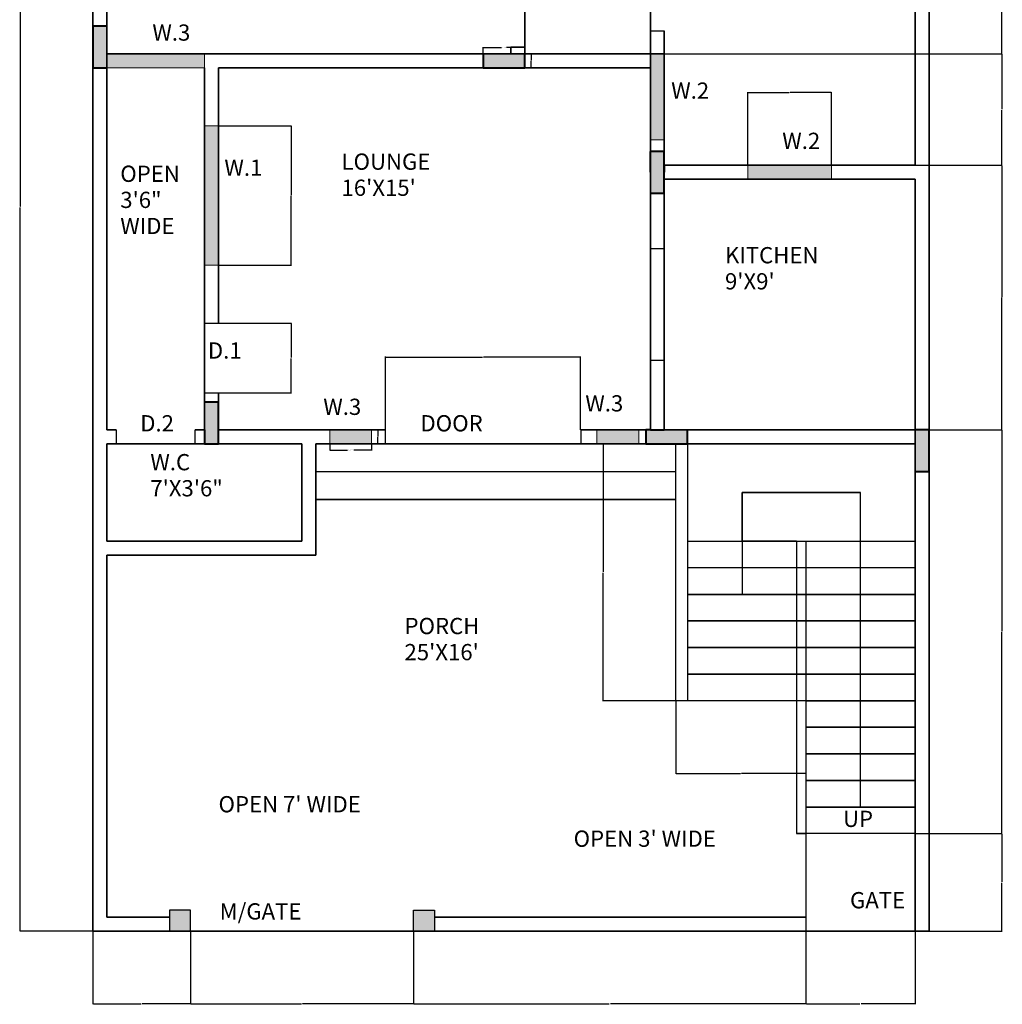
# Model space of a CAD drawing. Units: inches. Extents: x 2156 to 3149, y 1513 to 2286.
# Tile 1 of 5: x 2156 to 2579, y 1513 to 1937. Entities that reach past the tile are written whole.
import ezdxf

# ---------------------------------------------------------------- set-up
doc = ezdxf.new("R2010")
doc.units = ezdxf.units.IN
for name, color, linetype, lineweight in [('A-ANNO-DIMS', 2, 'Continuous', 18), ('A-ANNO-TEXT', 7, 'Continuous', 18), ('A-AREA-IDEN', 7, 'Continuous', 18), ('A-COLS', 7, 'Continuous', 40), ('A-COLS-PATT', 18, 'Continuous', 13), ('A-CONS', 8, 'Continuous', 9), ('A-DOOR', 3, 'Continuous', 25), ('A-FLOR-STRS', 7, 'Continuous', 25), ('A-GLAZ', 4, 'Continuous', 18), ('A-GLAZ-PATT', 252, 'Continuous', 13), ('A-SITE-GATE', 3, 'Continuous', 25), ('A-SITE-WALL', 7, 'Continuous', 35), ('A-WALL', 7, 'Continuous', 35)]:
    doc.layers.add(name, color=color, linetype=linetype, lineweight=lineweight)
doc.styles.get("Standard").update_dxf_attribs({"font": 'arial.ttf'})
doc.dimstyles.get("Standard").update_dxf_attribs({"dimtxt": 0.18, "dimasz": 0.18, "dimexe": 0.18, "dimexo": 0.0625, "dimgap": 0.09, "dimtad": 0, "dimtih": 1, "dimtoh": 1, "dimdec": 4, "dimzin": 0, "dimdsep": 46, "dimtxsty": 'Standard', "dimcen": 0.09, "dimadec": 0, "dimazin": 0, "dimtfac": 1, "dimtdec": 4, "dimtofl": 0, "dimtmove": 0, "dimatfit": 3, "dimfxl": 1, "dimtolj": 1, "dimtzin": 0, "dimarcsym": 0})

# ---------------------------------------------------------------- blocks, each defined once
blk = doc.blocks.new('COL-6X18-PLAN')
for p, q in [((6, 18), (0, 18)), ((0, 18), (0, 0)), ((0, 0), (6, 0))]:
    blk.add_line(p, q)
blk = doc.blocks.new('WIN-W3-18-PLAN')
for p, q in [((18, 6), (0, 6)), ((0, 6), (0, 0)), ((18, 0), (18, 6))]:
    blk.add_line(p, q)
blk = doc.blocks.new('*D7')
at = {"layer": 'A-ANNO-DIMS', "color": 0, "lineweight": -2, "transparency": 16777216}
for p, q in [((2355.92, 1922.6), (2355.92, 1925.42)), ((2356.1, 1925.24), (2363.81, 1925.24)), ((2373.74, 1925.24), (2366.03, 1925.24)), ((2373.92, 1922.6), (2373.92, 1925.42))]:
    blk.add_line(p, q, dxfattribs=at)
at = {"layer": 'A-ANNO-DIMS', "color": 0, "transparency": 16777216}
for points in [[(2356.1, 1925.27), (2356.1, 1925.21), (2355.92, 1925.24)], [(2373.74, 1925.27), (2373.74, 1925.21), (2373.92, 1925.24)]]:
    blk.add_solid(points, dxfattribs=at)
at = {"layer": 'Defpoints', "color": 0, "transparency": 16777216}
for p in [(2355.92, 1925.24), (2355.92, 1922.54), (2373.92, 1922.54)]:
    blk.add_point(p, dxfattribs=at)
at = {"layer": 'A-ANNO-DIMS', "color": 0, "transparency": 16777216, "insert": (2364.92, 1925.24), "char_height": 0.18, "attachment_point": 5}
blk.add_mtext('\\A1;COLUMN 18 TYP.', dxfattribs=at)
blk = doc.blocks.new('*D8')
at = {"layer": 'A-ANNO-DIMS', "color": 0, "lineweight": -2, "transparency": 16777216}
for p, q in [((2373.98, 1922.54), (2376.8, 1922.54)), ((2376.62, 1922.36), (2376.62, 1919.72)), ((2376.62, 1916.72), (2376.62, 1919.35)), ((2373.98, 1916.54), (2376.8, 1916.54))]:
    blk.add_line(p, q, dxfattribs=at)
at = {"layer": 'A-ANNO-DIMS', "color": 0, "transparency": 16777216}
for points in [[(2376.59, 1922.36), (2376.65, 1922.36), (2376.62, 1922.54)], [(2376.59, 1916.72), (2376.65, 1916.72), (2376.62, 1916.54)]]:
    blk.add_solid(points, dxfattribs=at)
at = {"layer": 'Defpoints', "color": 0, "transparency": 16777216}
for p in [(2373.92, 1922.54), (2376.62, 1922.54), (2373.92, 1916.54)]:
    blk.add_point(p, dxfattribs=at)
at = {"layer": 'A-ANNO-DIMS', "color": 0, "transparency": 16777216, "insert": (2376.62, 1919.54), "char_height": 0.18, "attachment_point": 5}
blk.add_mtext('\\A1;6 TYP.', dxfattribs=at)
blk = doc.blocks.new('*D11')
at = {"layer": 'A-ANNO-DIMS', "color": 0, "lineweight": -2, "transparency": 16777216}
for p, q in [((2289.92, 1754.47), (2289.92, 1751.66)), ((2307.92, 1754.47), (2307.92, 1751.66)), ((2290.1, 1751.84), (2297.58, 1751.84)), ((2307.74, 1751.84), (2300.26, 1751.84))]:
    blk.add_line(p, q, dxfattribs=at)
at = {"layer": 'A-ANNO-DIMS', "color": 0, "transparency": 16777216}
for points in [[(2290.1, 1751.87), (2290.1, 1751.81), (2289.92, 1751.84)], [(2307.74, 1751.87), (2307.74, 1751.81), (2307.92, 1751.84)]]:
    blk.add_solid(points, dxfattribs=at)
at = {"layer": 'Defpoints', "color": 0, "transparency": 16777216}
for p in [(2289.92, 1754.54), (2307.92, 1754.54), (2307.92, 1751.84)]:
    blk.add_point(p, dxfattribs=at)
at = {"layer": 'A-ANNO-DIMS', "color": 0, "transparency": 16777216, "insert": (2298.92, 1751.84), "char_height": 0.18, "attachment_point": 5}
blk.add_mtext('\\A1;W3 WINDOW 18 TYP.', dxfattribs=at)
blk = doc.blocks.new('*D12')
at = {"layer": 'A-ANNO-DIMS', "color": 0, "lineweight": -2, "transparency": 16777216}
for p, q in [((2307.98, 1760.54), (2310.8, 1760.54)), ((2310.62, 1760.36), (2310.62, 1757.72)), ((2310.62, 1754.72), (2310.62, 1757.35)), ((2307.98, 1754.54), (2310.8, 1754.54))]:
    blk.add_line(p, q, dxfattribs=at)
at = {"layer": 'A-ANNO-DIMS', "color": 0, "transparency": 16777216}
for points in [[(2310.59, 1760.36), (2310.65, 1760.36), (2310.62, 1760.54)], [(2310.59, 1754.72), (2310.65, 1754.72), (2310.62, 1754.54)]]:
    blk.add_solid(points, dxfattribs=at)
at = {"layer": 'Defpoints', "color": 0, "transparency": 16777216}
for p in [(2307.92, 1760.54), (2310.62, 1760.54), (2307.92, 1754.54)]:
    blk.add_point(p, dxfattribs=at)
at = {"layer": 'A-ANNO-DIMS', "color": 0, "transparency": 16777216, "insert": (2310.62, 1757.54), "char_height": 0.18, "attachment_point": 5}
blk.add_mtext('\\A1;6 TYP.', dxfattribs=at)
blk = doc.blocks.new('*D20')
at = {"layer": 'A-ANNO-DIMS', "color": 0, "lineweight": -2, "transparency": 16777216}
for p, q in [((2187.92, 1544.47), (2187.92, 1513.01)), ((2229.92, 1544.47), (2229.92, 1513.01)), ((2188.1, 1513.19), (2208.7, 1513.19)), ((2229.74, 1513.19), (2209.14, 1513.19))]:
    blk.add_line(p, q, dxfattribs=at)
at = {"layer": 'A-ANNO-DIMS', "color": 0, "transparency": 16777216}
for points in [[(2188.1, 1513.22), (2188.1, 1513.16), (2187.92, 1513.19)], [(2229.74, 1513.22), (2229.74, 1513.16), (2229.92, 1513.19)]]:
    blk.add_solid(points, dxfattribs=at)
at = {"layer": 'Defpoints', "color": 0, "transparency": 16777216}
for p in [(2187.92, 1544.54), (2229.92, 1544.54), (2229.92, 1513.19)]:
    blk.add_point(p, dxfattribs=at)
at = {"layer": 'A-ANNO-DIMS', "color": 0, "transparency": 16777216, "insert": (2208.92, 1513.19), "char_height": 0.18, "attachment_point": 5}
blk.add_mtext('\\A1;42', dxfattribs=at)
blk = doc.blocks.new('*D21')
at = {"layer": 'A-ANNO-DIMS', "color": 0, "lineweight": -2, "transparency": 16777216}
for p, q in [((2229.92, 1544.47), (2229.92, 1513.01)), ((2325.92, 1544.47), (2325.92, 1513.01)), ((2230.1, 1513.19), (2277.7, 1513.19)), ((2325.74, 1513.19), (2278.14, 1513.19))]:
    blk.add_line(p, q, dxfattribs=at)
at = {"layer": 'A-ANNO-DIMS', "color": 0, "transparency": 16777216}
for points in [[(2230.1, 1513.22), (2230.1, 1513.16), (2229.92, 1513.19)], [(2325.74, 1513.22), (2325.74, 1513.16), (2325.92, 1513.19)]]:
    blk.add_solid(points, dxfattribs=at)
at = {"layer": 'Defpoints', "color": 0, "transparency": 16777216}
for p in [(2229.92, 1544.54), (2325.92, 1544.54), (2325.92, 1513.19)]:
    blk.add_point(p, dxfattribs=at)
at = {"layer": 'A-ANNO-DIMS', "color": 0, "transparency": 16777216, "insert": (2277.92, 1513.19), "char_height": 0.18, "attachment_point": 5}
blk.add_mtext('\\A1;96', dxfattribs=at)
blk = doc.blocks.new('*D22')
at = {"layer": 'A-ANNO-DIMS', "color": 0, "lineweight": -2, "transparency": 16777216}
for p, q in [((2325.92, 1544.47), (2325.92, 1513.01)), ((2494.92, 1544.47), (2494.92, 1513.01)), ((2326.1, 1513.19), (2410.14, 1513.19)), ((2494.74, 1513.19), (2410.7, 1513.19))]:
    blk.add_line(p, q, dxfattribs=at)
at = {"layer": 'A-ANNO-DIMS', "color": 0, "transparency": 16777216}
for points in [[(2326.1, 1513.22), (2326.1, 1513.16), (2325.92, 1513.19)], [(2494.74, 1513.22), (2494.74, 1513.16), (2494.92, 1513.19)]]:
    blk.add_solid(points, dxfattribs=at)
at = {"layer": 'Defpoints', "color": 0, "transparency": 16777216}
for p in [(2325.92, 1544.54), (2494.92, 1544.54), (2494.92, 1513.19)]:
    blk.add_point(p, dxfattribs=at)
at = {"layer": 'A-ANNO-DIMS', "color": 0, "transparency": 16777216, "insert": (2410.42, 1513.19), "char_height": 0.18, "attachment_point": 5}
blk.add_mtext('\\A1;169', dxfattribs=at)
blk = doc.blocks.new('*D23')
at = {"layer": 'A-ANNO-DIMS', "color": 0, "lineweight": -2, "transparency": 16777216}
for p, q in [((2494.92, 1544.47), (2494.92, 1513.01)), ((2541.92, 1544.47), (2541.92, 1513.01)), ((2495.1, 1513.19), (2518.2, 1513.19)), ((2541.74, 1513.19), (2518.64, 1513.19))]:
    blk.add_line(p, q, dxfattribs=at)
at = {"layer": 'A-ANNO-DIMS', "color": 0, "transparency": 16777216}
for points in [[(2495.1, 1513.22), (2495.1, 1513.16), (2494.92, 1513.19)], [(2541.74, 1513.22), (2541.74, 1513.16), (2541.92, 1513.19)]]:
    blk.add_solid(points, dxfattribs=at)
at = {"layer": 'Defpoints', "color": 0, "transparency": 16777216}
for p in [(2494.92, 1544.54), (2541.92, 1544.54), (2541.92, 1513.19)]:
    blk.add_point(p, dxfattribs=at)
at = {"layer": 'A-ANNO-DIMS', "color": 0, "transparency": 16777216, "insert": (2518.42, 1513.19), "char_height": 0.18, "attachment_point": 5}
blk.add_mtext('\\A1;47', dxfattribs=at)
blk = doc.blocks.new('*D24')
at = {"layer": 'A-ANNO-DIMS', "color": 0, "lineweight": -2, "transparency": 16777216}
for p, q in [((2187.86, 2168.54), (2156.39, 2168.54)), ((2156.57, 2168.36), (2156.57, 1856.72)), ((2156.57, 1544.72), (2156.57, 1856.35)), ((2187.86, 1544.54), (2156.39, 1544.54))]:
    blk.add_line(p, q, dxfattribs=at)
at = {"layer": 'A-ANNO-DIMS', "color": 0, "transparency": 16777216}
for points in [[(2156.54, 2168.36), (2156.6, 2168.36), (2156.57, 2168.54)], [(2156.54, 1544.72), (2156.6, 1544.72), (2156.57, 1544.54)]]:
    blk.add_solid(points, dxfattribs=at)
at = {"layer": 'Defpoints', "color": 0, "transparency": 16777216}
for p in [(2156.57, 2168.54), (2187.92, 2168.54), (2187.92, 1544.54)]:
    blk.add_point(p, dxfattribs=at)
at = {"layer": 'A-ANNO-DIMS', "color": 0, "transparency": 16777216, "insert": (2156.57, 1856.54), "char_height": 0.18, "attachment_point": 5}
blk.add_mtext('\\A1;624', dxfattribs=at)
blk = doc.blocks.new('*D25')
at = {"layer": 'A-ANNO-DIMS', "color": 0, "lineweight": -2, "transparency": 16777216}
for p, q in [((2541.98, 1586.54), (2579.45, 1586.54)), ((2579.27, 1586.36), (2579.27, 1565.72)), ((2579.27, 1544.72), (2579.27, 1565.36)), ((2547.98, 1544.54), (2579.45, 1544.54))]:
    blk.add_line(p, q, dxfattribs=at)
at = {"layer": 'A-ANNO-DIMS', "color": 0, "transparency": 16777216}
for points in [[(2579.24, 1586.36), (2579.3, 1586.36), (2579.27, 1586.54)], [(2579.24, 1544.72), (2579.3, 1544.72), (2579.27, 1544.54)]]:
    blk.add_solid(points, dxfattribs=at)
at = {"layer": 'Defpoints', "color": 0, "transparency": 16777216}
for p in [(2541.92, 1586.54), (2579.27, 1586.54), (2547.92, 1544.54)]:
    blk.add_point(p, dxfattribs=at)
at = {"layer": 'A-ANNO-DIMS', "color": 0, "transparency": 16777216, "insert": (2579.27, 1565.54), "char_height": 0.18, "attachment_point": 5}
blk.add_mtext('\\A1;42', dxfattribs=at)
blk = doc.blocks.new('*D26')
at = {"layer": 'A-ANNO-DIMS', "color": 0, "lineweight": -2, "transparency": 16777216}
for p, q in [((2547.98, 1760.54), (2579.45, 1760.54)), ((2579.27, 1760.36), (2579.27, 1673.72)), ((2579.27, 1586.72), (2579.27, 1673.36)), ((2541.98, 1586.54), (2579.45, 1586.54))]:
    blk.add_line(p, q, dxfattribs=at)
at = {"layer": 'A-ANNO-DIMS', "color": 0, "transparency": 16777216}
for points in [[(2579.24, 1760.36), (2579.3, 1760.36), (2579.27, 1760.54)], [(2579.24, 1586.72), (2579.3, 1586.72), (2579.27, 1586.54)]]:
    blk.add_solid(points, dxfattribs=at)
at = {"layer": 'Defpoints', "color": 0, "transparency": 16777216}
for p in [(2547.92, 1760.54), (2579.27, 1760.54), (2541.92, 1586.54)]:
    blk.add_point(p, dxfattribs=at)
at = {"layer": 'A-ANNO-DIMS', "color": 0, "transparency": 16777216, "insert": (2579.27, 1673.54), "char_height": 0.18, "attachment_point": 5}
blk.add_mtext('\\A1;174', dxfattribs=at)
blk = doc.blocks.new('*D27')
at = {"layer": 'A-ANNO-DIMS', "color": 0, "lineweight": -2, "transparency": 16777216}
for p, q in [((2541.98, 1874.54), (2579.45, 1874.54)), ((2579.27, 1874.36), (2579.27, 1817.72)), ((2579.27, 1760.72), (2579.27, 1817.36)), ((2547.98, 1760.54), (2579.45, 1760.54))]:
    blk.add_line(p, q, dxfattribs=at)
at = {"layer": 'A-ANNO-DIMS', "color": 0, "transparency": 16777216}
for points in [[(2579.24, 1874.36), (2579.3, 1874.36), (2579.27, 1874.54)], [(2579.24, 1760.72), (2579.3, 1760.72), (2579.27, 1760.54)]]:
    blk.add_solid(points, dxfattribs=at)
at = {"layer": 'Defpoints', "color": 0, "transparency": 16777216}
for p in [(2541.92, 1874.54), (2579.27, 1874.54), (2547.92, 1760.54)]:
    blk.add_point(p, dxfattribs=at)
at = {"layer": 'A-ANNO-DIMS', "color": 0, "transparency": 16777216, "insert": (2579.27, 1817.54), "char_height": 0.18, "attachment_point": 5}
blk.add_mtext('\\A1;114', dxfattribs=at)
blk = doc.blocks.new('*D28')
at = {"layer": 'A-ANNO-DIMS', "color": 0, "lineweight": -2, "transparency": 16777216}
for p, q in [((2433.98, 1922.54), (2579.45, 1922.54)), ((2579.27, 1922.36), (2579.27, 1898.72)), ((2579.27, 1874.72), (2579.27, 1898.35)), ((2541.98, 1874.54), (2579.45, 1874.54))]:
    blk.add_line(p, q, dxfattribs=at)
at = {"layer": 'A-ANNO-DIMS', "color": 0, "transparency": 16777216}
for points in [[(2579.24, 1922.36), (2579.3, 1922.36), (2579.27, 1922.54)], [(2579.24, 1874.72), (2579.3, 1874.72), (2579.27, 1874.54)]]:
    blk.add_solid(points, dxfattribs=at)
at = {"layer": 'Defpoints', "color": 0, "transparency": 16777216}
for p in [(2433.92, 1922.54), (2579.27, 1922.54), (2541.92, 1874.54)]:
    blk.add_point(p, dxfattribs=at)
at = {"layer": 'A-ANNO-DIMS', "color": 0, "transparency": 16777216, "insert": (2579.27, 1898.54), "char_height": 0.18, "attachment_point": 5}
blk.add_mtext('\\A1;48', dxfattribs=at)
blk = doc.blocks.new('*D29')
at = {"layer": 'A-ANNO-DIMS', "color": 0, "lineweight": -2, "transparency": 16777216}
for p, q in [((2547.98, 1988.54), (2579.45, 1988.54)), ((2579.27, 1988.36), (2579.27, 1955.72)), ((2579.27, 1922.72), (2579.27, 1955.35)), ((2433.98, 1922.54), (2579.45, 1922.54))]:
    blk.add_line(p, q, dxfattribs=at)
at = {"layer": 'A-ANNO-DIMS', "color": 0, "transparency": 16777216}
for points in [[(2579.24, 1988.36), (2579.3, 1988.36), (2579.27, 1988.54)], [(2579.24, 1922.72), (2579.3, 1922.72), (2579.27, 1922.54)]]:
    blk.add_solid(points, dxfattribs=at)
at = {"layer": 'Defpoints', "color": 0, "transparency": 16777216}
for p in [(2547.92, 1988.54), (2579.27, 1988.54), (2433.92, 1922.54)]:
    blk.add_point(p, dxfattribs=at)
at = {"layer": 'A-ANNO-DIMS', "color": 0, "transparency": 16777216, "insert": (2579.27, 1955.54), "char_height": 0.18, "attachment_point": 5}
blk.add_mtext('\\A1;66', dxfattribs=at)
blk = doc.blocks.new('*D39')
at = {"layer": 'A-ANNO-DIMS', "color": 0, "lineweight": -2, "transparency": 16777216}
for p, q in [((2241.98, 1891.54), (2273.45, 1891.54)), ((2273.27, 1891.36), (2273.27, 1861.72)), ((2273.27, 1831.72), (2273.27, 1861.35)), ((2241.98, 1831.54), (2273.45, 1831.54))]:
    blk.add_line(p, q, dxfattribs=at)
at = {"layer": 'A-ANNO-DIMS', "color": 0, "transparency": 16777216}
for points in [[(2273.24, 1891.36), (2273.3, 1891.36), (2273.27, 1891.54)], [(2273.24, 1831.72), (2273.3, 1831.72), (2273.27, 1831.54)]]:
    blk.add_solid(points, dxfattribs=at)
at = {"layer": 'Defpoints', "color": 0, "transparency": 16777216}
for p in [(2241.92, 1891.54), (2241.92, 1831.54), (2273.27, 1831.54)]:
    blk.add_point(p, dxfattribs=at)
at = {"layer": 'A-ANNO-DIMS', "color": 0, "transparency": 16777216, "insert": (2273.27, 1861.54), "char_height": 0.18, "attachment_point": 5}
blk.add_mtext('\\A1;60', dxfattribs=at)
blk = doc.blocks.new('*D40')
at = {"layer": 'A-ANNO-DIMS', "color": 0, "lineweight": -2, "transparency": 16777216}
for p, q in [((2241.98, 1806.54), (2273.45, 1806.54)), ((2273.27, 1806.36), (2273.27, 1791.72)), ((2273.27, 1776.72), (2273.27, 1791.35)), ((2241.98, 1776.54), (2273.45, 1776.54))]:
    blk.add_line(p, q, dxfattribs=at)
at = {"layer": 'A-ANNO-DIMS', "color": 0, "transparency": 16777216}
for points in [[(2273.24, 1806.36), (2273.3, 1806.36), (2273.27, 1806.54)], [(2273.24, 1776.72), (2273.3, 1776.72), (2273.27, 1776.54)]]:
    blk.add_solid(points, dxfattribs=at)
at = {"layer": 'Defpoints', "color": 0, "transparency": 16777216}
for p in [(2241.92, 1806.54), (2241.92, 1776.54), (2273.27, 1776.54)]:
    blk.add_point(p, dxfattribs=at)
at = {"layer": 'A-ANNO-DIMS', "color": 0, "transparency": 16777216, "insert": (2273.27, 1791.54), "char_height": 0.18, "attachment_point": 5}
blk.add_mtext('\\A1;30', dxfattribs=at)
blk = doc.blocks.new('*D41')
at = {"layer": 'A-ANNO-DIMS', "color": 0, "lineweight": -2, "transparency": 16777216}
for p, q in [((2313.92, 1760.6), (2313.92, 1792.07)), ((2314.1, 1791.89), (2355.7, 1791.89)), ((2397.74, 1791.89), (2356.14, 1791.89)), ((2397.92, 1760.6), (2397.92, 1792.07))]:
    blk.add_line(p, q, dxfattribs=at)
at = {"layer": 'A-ANNO-DIMS', "color": 0, "transparency": 16777216}
for points in [[(2314.1, 1791.92), (2314.1, 1791.86), (2313.92, 1791.89)], [(2397.74, 1791.92), (2397.74, 1791.86), (2397.92, 1791.89)]]:
    blk.add_solid(points, dxfattribs=at)
at = {"layer": 'Defpoints', "color": 0, "transparency": 16777216}
for p in [(2397.92, 1791.89), (2313.92, 1760.54), (2397.92, 1760.54)]:
    blk.add_point(p, dxfattribs=at)
at = {"layer": 'A-ANNO-DIMS', "color": 0, "transparency": 16777216, "insert": (2355.92, 1791.89), "char_height": 0.18, "attachment_point": 5}
blk.add_mtext('\\A1;84', dxfattribs=at)
blk = doc.blocks.new('*D42')
at = {"layer": 'A-ANNO-DIMS', "color": 0, "lineweight": -2, "transparency": 16777216}
for p, q in [((2469.92, 1874.6), (2469.92, 1906.07)), ((2470.1, 1905.89), (2487.7, 1905.89)), ((2505.74, 1905.89), (2488.14, 1905.89)), ((2505.92, 1874.6), (2505.92, 1906.07))]:
    blk.add_line(p, q, dxfattribs=at)
at = {"layer": 'A-ANNO-DIMS', "color": 0, "transparency": 16777216}
for points in [[(2470.1, 1905.92), (2470.1, 1905.86), (2469.92, 1905.89)], [(2505.74, 1905.92), (2505.74, 1905.86), (2505.92, 1905.89)]]:
    blk.add_solid(points, dxfattribs=at)
at = {"layer": 'Defpoints', "color": 0, "transparency": 16777216}
for p in [(2505.92, 1905.89), (2469.92, 1874.54), (2505.92, 1874.54)]:
    blk.add_point(p, dxfattribs=at)
at = {"layer": 'A-ANNO-DIMS', "color": 0, "transparency": 16777216, "insert": (2487.92, 1905.89), "char_height": 0.18, "attachment_point": 5}
blk.add_mtext('\\A1;36', dxfattribs=at)
blk = doc.blocks.new('*D43')
at = {"layer": 'A-ANNO-DIMS', "color": 0, "lineweight": -2, "transparency": 16777216}
for p, q in [((2438.86, 1754.54), (2407.39, 1754.54)), ((2407.57, 1754.36), (2407.57, 1699.35)), ((2407.57, 1643.99), (2407.57, 1698.99)), ((2438.86, 1643.81), (2407.39, 1643.81))]:
    blk.add_line(p, q, dxfattribs=at)
at = {"layer": 'A-ANNO-DIMS', "color": 0, "transparency": 16777216}
for points in [[(2407.54, 1754.36), (2407.6, 1754.36), (2407.57, 1754.54)], [(2407.54, 1643.99), (2407.6, 1643.99), (2407.57, 1643.81)]]:
    blk.add_solid(points, dxfattribs=at)
at = {"layer": 'Defpoints', "color": 0, "transparency": 16777216}
for p in [(2407.57, 1754.54), (2438.92, 1754.54), (2438.92, 1643.81)]:
    blk.add_point(p, dxfattribs=at)
at = {"layer": 'A-ANNO-DIMS', "color": 0, "transparency": 16777216, "insert": (2407.57, 1699.17), "char_height": 0.18, "attachment_point": 5}
blk.add_mtext('\\A1;110.73', dxfattribs=at)
blk = doc.blocks.new('*D44')
at = {"layer": 'A-ANNO-DIMS', "color": 0, "lineweight": -2, "transparency": 16777216}
for p, q in [((2438.92, 1643.75), (2438.92, 1612.28)), ((2494.92, 1643.75), (2494.92, 1612.28)), ((2439.1, 1612.46), (2466.7, 1612.46)), ((2494.74, 1612.46), (2467.14, 1612.46))]:
    blk.add_line(p, q, dxfattribs=at)
at = {"layer": 'A-ANNO-DIMS', "color": 0, "transparency": 16777216}
for points in [[(2439.1, 1612.49), (2439.1, 1612.43), (2438.92, 1612.46)], [(2494.74, 1612.49), (2494.74, 1612.43), (2494.92, 1612.46)]]:
    blk.add_solid(points, dxfattribs=at)
at = {"layer": 'Defpoints', "color": 0, "transparency": 16777216}
for p in [(2438.92, 1643.81), (2494.92, 1643.81), (2438.92, 1612.46)]:
    blk.add_point(p, dxfattribs=at)
at = {"layer": 'A-ANNO-DIMS', "color": 0, "transparency": 16777216, "insert": (2466.92, 1612.46), "char_height": 0.18, "attachment_point": 5}
blk.add_mtext('\\A1;56', dxfattribs=at)

msp = doc.modelspace()

# ---------------------------------------------------------------- hatches: boundary and pattern name
at = {"layer": 'A-COLS-PATT'}
h = msp.add_hatch(color=256, dxfattribs=at)
h.dxf.hatch_style = 1
h.paths.add_polyline_path([(2193.921, 2120.536), (2193.921, 2126.536), (2187.921, 2126.536), (2187.921, 2108.536), (2193.921, 2108.536)])
h.paths.add_polyline_path([(2385.921, 2126.536), (2367.921, 2126.536), (2367.921, 2120.536), (2373.921, 2120.536), (2385.921, 2120.536)])
h.paths.add_polyline_path([(2547.921, 2126.536), (2541.921, 2126.536), (2541.921, 2108.536), (2547.921, 2108.536)])
h.paths.add_polyline_path([(2547.921, 1988.536), (2541.921, 1988.536), (2541.921, 1982.536), (2547.921, 1982.536)])
h.paths.add_polyline_path([(2541.921, 1988.536), (2529.921, 1988.536), (2529.921, 1982.536), (2541.921, 1982.536)])
h.paths.add_polyline_path([(2373.921, 1922.536), (2367.921, 1922.536), (2355.921, 1922.536), (2355.921, 1916.536), (2373.921, 1916.536)])
h.paths.add_polyline_path([(2193.921, 1934.536), (2187.921, 1934.536), (2187.921, 1916.536), (2193.921, 1916.536)])
h.paths.add_polyline_path([(2433.921, 1880.536), (2427.921, 1880.536), (2427.921, 1871.536), (2427.921, 1862.536), (2433.921, 1862.536)])
h.paths.add_polyline_path([(2241.921, 1772.536), (2235.921, 1772.536), (2235.921, 1760.536), (2235.921, 1754.536), (2241.921, 1754.536)])
h.paths.add_polyline_path([(2443.921, 1760.536), (2433.921, 1760.536), (2427.921, 1760.536), (2425.921, 1760.536), (2425.921, 1754.536), (2443.921, 1754.536)])
h.paths.add_polyline_path([(2547.921, 1760.536), (2541.921, 1760.536), (2541.921, 1754.536), (2541.921, 1742.536), (2547.921, 1742.536)])
h = msp.add_hatch(color=256, dxfattribs=at)
h.dxf.hatch_style = 1
h.paths.add_polyline_path([(2334.921, 1553.536), (2325.921, 1553.536), (2325.921, 1550.536), (2325.921, 1544.536), (2334.921, 1544.536)])
h.paths.add_polyline_path([(2229.921, 1553.536), (2220.921, 1553.536), (2220.921, 1544.536), (2229.921, 1544.536)])
at = {"layer": 'A-GLAZ-PATT'}
h = msp.add_hatch(color=256, dxfattribs=at)
h.dxf.hatch_style = 1
h.paths.add_polyline_path([(2490.921, 2126.536), (2397.921, 2126.536), (2397.921, 2120.536), (2490.921, 2120.536)])
h.paths.add_polyline_path([(2337.921, 2126.536), (2313.921, 2126.536), (2313.921, 2120.536), (2325.921, 2120.536), (2337.921, 2120.536)])
h.paths.add_polyline_path([(2247.921, 2126.536), (2223.921, 2126.536), (2223.921, 2120.536), (2235.921, 2120.536), (2247.921, 2120.536)])
h.paths.add_polyline_path([(2241.921, 1891.536), (2235.921, 1891.536), (2235.921, 1831.536), (2241.921, 1831.536), (2241.921, 1861.536)])
h.paths.add_polyline_path([(2235.921, 1922.536), (2193.921, 1922.536), (2193.921, 1916.536), (2235.921, 1916.536)])
h.paths.add_polyline_path([(2505.921, 1874.536), (2469.921, 1874.536), (2469.921, 1868.536), (2505.921, 1868.536)])
h.paths.add_polyline_path([(2523.921, 1988.536), (2451.921, 1988.536), (2451.921, 1982.536), (2523.921, 1982.536)])
h.paths.add_polyline_path([(2307.921, 1760.536), (2289.921, 1760.536), (2289.921, 1754.536), (2298.921, 1754.536), (2307.921, 1754.536)])
h.paths.add_polyline_path([(2422.921, 1760.536), (2404.921, 1760.536), (2404.921, 1754.536), (2413.921, 1754.536), (2422.921, 1754.536)])
h = msp.add_hatch(color=256, dxfattribs=at)
h.dxf.hatch_style = 1
h.paths.add_polyline_path([(2433.921, 1922.536), (2427.921, 1922.536), (2427.921, 1916.536), (2427.921, 1885.536), (2433.921, 1885.536)])

# ---------------------------------------------------------------- linework, layer by layer
at = {"layer": 'A-COLS'}
for p, q in [((2427.921, 1871.536), (2427.921, 1880.536)), ((2427.921, 1871.536), (2427.921, 1871.536)), ((2433.921, 1868.536), (2433.921, 1874.536)), ((2433.921, 1874.536), (2433.921, 1871.536)), ((2235.921, 1760.536), (2235.921, 1754.536)), ((2427.921, 1760.536), (2425.921, 1760.536)), ((2427.921, 1760.536), (2433.921, 1760.536)), ((2541.921, 1742.536), (2547.921, 1742.536))]:
    msp.add_line(p, q, dxfattribs=at)
at = {"layer": 'A-CONS'}
for p in [(2541.921, 1701.081), (2541.921, 1689.627), (2541.921, 1678.172), (2541.921, 1666.717), (2541.921, 1655.263), (2541.921, 1643.808), (2541.921, 1632.354), (2541.921, 1620.899), (2541.921, 1609.445), (2541.921, 1597.99)]:
    msp.add_point(p, dxfattribs=at)
at = {"layer": 'A-DOOR'}
for p, q in [((2373.921, 1925.536), (2373.921, 1961.536)), ((2427.921, 1932.536), (2433.921, 1932.536)), ((2367.921, 1925.536), (2373.921, 1925.536)), ((2433.921, 1838.536), (2427.921, 1838.536)), ((2427.921, 1838.536), (2427.921, 1790.536)), ((2235.921, 1776.536), (2235.921, 1806.536)), ((2235.921, 1806.536), (2241.921, 1806.536)), ((2427.921, 1790.536), (2433.921, 1790.536)), ((2235.921, 1776.536), (2241.921, 1776.536)), ((2197.921, 1760.536), (2197.921, 1754.536)), ((2231.921, 1754.536), (2231.921, 1760.536)), ((2313.921, 1754.536), (2313.921, 1760.536)), ((2397.921, 1760.536), (2397.921, 1754.536))]:
    msp.add_line(p, q, dxfattribs=at)
at = {"layer": 'A-FLOR-STRS'}
for p, q in [((2283.921, 1730.536), (2283.921, 1754.536)), ((2283.921, 1754.536), (2283.921, 1742.536)), ((2438.921, 1643.808), (2438.921, 1754.536)), ((2443.921, 1754.536), (2443.921, 1643.808)), ((2443.921, 1754.536), (2443.921, 1712.536)), ((2283.921, 1742.536), (2438.921, 1742.536)), ((2467.421, 1712.536), (2467.421, 1733.536)), ((2467.421, 1733.536), (2518.421, 1733.536)), ((2518.421, 1733.536), (2467.421, 1733.536)), ((2467.421, 1733.536), (2467.421, 1712.536)), ((2518.421, 1712.536), (2518.421, 1733.536)), ((2283.921, 1706.536), (2283.921, 1730.536)), ((2283.921, 1730.536), (2438.921, 1730.536)), ((2438.921, 1730.536), (2283.921, 1730.536)), ((2443.921, 1712.536), (2541.921, 1712.536)), ((2443.921, 1712.536), (2490.921, 1712.536)), ((2490.921, 1712.536), (2467.421, 1712.536)), ((2467.421, 1712.536), (2467.421, 1689.627)), ((2490.921, 1712.536), (2490.921, 1606.981)), ((2494.921, 1712.536), (2494.921, 1606.981)), ((2518.421, 1597.99), (2518.421, 1712.536)), ((2541.921, 1712.536), (2541.921, 1586.536)), ((2541.921, 1701.081), (2443.921, 1701.081)), ((2541.921, 1689.627), (2541.921, 1701.081)), ((2541.921, 1689.627), (2443.921, 1689.627)), ((2443.921, 1689.627), (2541.921, 1689.627)), ((2541.921, 1678.172), (2541.921, 1689.627)), ((2541.921, 1678.172), (2443.921, 1678.172)), ((2443.921, 1678.172), (2541.921, 1678.172)), ((2541.921, 1678.172), (2494.921, 1678.172)), ((2494.921, 1678.172), (2541.921, 1678.172)), ((2541.921, 1666.717), (2541.921, 1678.172)), ((2494.921, 1666.717), (2443.921, 1666.717)), ((2443.921, 1666.717), (2494.921, 1666.717)), ((2541.921, 1666.717), (2494.921, 1666.717)), ((2494.921, 1666.717), (2541.921, 1666.717)), ((2494.921, 1666.717), (2494.921, 1655.263)), ((2541.921, 1655.263), (2541.921, 1666.717)), ((2494.921, 1655.263), (2443.921, 1655.263)), ((2443.921, 1655.263), (2494.921, 1655.263)), ((2541.921, 1655.263), (2494.921, 1655.263)), ((2494.921, 1655.263), (2541.921, 1655.263)), ((2494.921, 1655.263), (2494.921, 1643.808)), ((2541.921, 1643.808), (2541.921, 1655.263)), ((2443.921, 1643.808), (2438.921, 1643.808)), ((2494.921, 1643.808), (2443.921, 1643.808)), ((2541.921, 1643.808), (2494.921, 1643.808)), ((2494.921, 1643.808), (2541.921, 1643.808)), ((2541.921, 1632.354), (2541.921, 1643.808)), ((2541.921, 1632.354), (2494.921, 1632.354)), ((2494.921, 1632.354), (2541.921, 1632.354)), ((2541.921, 1620.899), (2541.921, 1632.354)), ((2541.921, 1620.899), (2494.921, 1620.899)), ((2494.921, 1620.899), (2541.921, 1620.899)), ((2541.921, 1609.445), (2541.921, 1620.899)), ((2541.921, 1609.445), (2494.921, 1609.445)), ((2494.921, 1609.445), (2541.921, 1609.445)), ((2541.921, 1597.99), (2541.921, 1609.445)), ((2490.921, 1606.981), (2490.921, 1586.536)), ((2494.921, 1606.981), (2494.921, 1586.536)), ((2541.921, 1597.99), (2494.921, 1597.99)), ((2494.921, 1597.99), (2541.921, 1597.99)), ((2541.921, 1586.536), (2490.921, 1586.536)), ((2490.921, 1586.536), (2494.921, 1586.536))]:
    msp.add_line(p, q, dxfattribs=at)
at = {"layer": 'A-GLAZ'}
for p, q in [((2193.921, 1922.536), (2193.921, 1916.536)), ((2235.921, 1916.536), (2235.921, 1922.536)), ((2193.921, 1916.536), (2235.921, 1916.536)), ((2235.921, 1831.536), (2235.921, 1891.536)), ((2235.921, 1891.536), (2241.921, 1891.536)), ((2427.921, 1885.536), (2433.921, 1885.536)), ((2469.921, 1874.536), (2469.921, 1868.536)), ((2505.921, 1868.536), (2505.921, 1874.536)), ((2469.921, 1868.536), (2505.921, 1868.536)), ((2241.921, 1831.536), (2235.921, 1831.536))]:
    msp.add_line(p, q, dxfattribs=at)
at = {"layer": 'A-SITE-GATE'}
for p, q in [((2494.921, 1586.536), (2494.921, 1544.536)), ((2229.921, 1553.536), (2220.921, 1553.536)), ((2220.921, 1553.536), (2220.921, 1544.536)), ((2229.921, 1544.536), (2229.921, 1553.536)), ((2325.921, 1550.536), (2325.921, 1553.536)), ((2325.921, 1553.536), (2334.921, 1553.536)), ((2334.921, 1553.536), (2334.921, 1544.536)), ((2220.921, 1550.536), (2220.921, 1544.536)), ((2325.921, 1544.536), (2325.921, 1550.536)), ((2220.921, 1544.536), (2229.921, 1544.536)), ((2334.921, 1544.536), (2325.921, 1544.536))]:
    msp.add_line(p, q, dxfattribs=at)
at = {"layer": 'A-SITE-WALL'}
for p, q in [((2187.921, 1544.536), (2187.921, 2168.536)), ((2547.921, 2168.536), (2547.921, 1544.536)), ((2541.921, 1868.536), (2541.921, 1544.536)), ((2193.921, 1550.536), (2193.921, 1706.536)), ((2541.921, 1550.536), (2541.921, 1586.536)), ((2193.921, 1550.536), (2220.921, 1550.536)), ((2220.921, 1550.536), (2193.921, 1550.536)), ((2494.921, 1550.536), (2334.921, 1550.536)), ((2541.921, 1544.536), (2541.921, 1550.536)), ((2547.921, 1544.536), (2187.921, 1544.536))]:
    msp.add_line(p, q, dxfattribs=at)
at = {"layer": 'A-WALL'}
for p, q in [((2193.921, 1760.536), (2193.921, 2054.536)), ((2373.921, 1982.536), (2373.921, 1922.536)), ((2427.921, 1922.536), (2427.921, 1982.536)), ((2541.921, 1982.536), (2541.921, 1874.536)), ((2427.921, 1922.536), (2427.921, 1932.536)), ((2433.921, 1932.536), (2433.921, 1874.536)), ((2367.921, 1922.536), (2193.921, 1922.536)), ((2367.921, 1922.536), (2367.921, 1925.536)), ((2367.921, 1925.536), (2367.921, 1922.536)), ((2373.921, 1922.536), (2367.921, 1922.536)), ((2373.921, 1922.536), (2433.921, 1922.536)), ((2433.921, 1922.536), (2427.921, 1922.536)), ((2427.921, 1916.536), (2427.921, 1922.536)), ((2235.921, 1916.536), (2235.921, 1760.536)), ((2241.921, 1916.536), (2427.921, 1916.536)), ((2241.921, 1916.536), (2241.921, 1806.536)), ((2241.921, 1806.536), (2241.921, 1916.536)), ((2427.921, 1916.536), (2427.921, 1760.536)), ((2427.921, 1880.536), (2427.921, 1885.536)), ((2427.921, 1880.536), (2427.921, 1885.536)), ((2433.921, 1874.536), (2541.921, 1874.536)), ((2433.921, 1874.536), (2541.921, 1874.536)), ((2487.921, 1874.536), (2469.921, 1874.536)), ((2541.921, 1874.536), (2487.921, 1874.536)), ((2541.921, 1868.536), (2433.921, 1868.536)), ((2433.921, 1868.536), (2433.921, 1760.536)), ((2433.921, 1760.536), (2433.921, 1862.536)), ((2433.921, 1862.536), (2433.921, 1814.536)), ((2241.921, 1806.536), (2241.921, 1861.536)), ((2241.921, 1861.536), (2241.921, 1831.536)), ((2433.921, 1814.536), (2433.921, 1838.536)), ((2235.921, 1772.536), (2235.921, 1776.536)), ((2241.921, 1760.536), (2241.921, 1776.536)), ((2193.921, 1760.536), (2197.921, 1760.536)), ((2193.921, 1760.536), (2197.921, 1760.536)), ((2231.921, 1760.536), (2235.921, 1760.536)), ((2313.921, 1760.536), (2241.921, 1760.536)), ((2427.921, 1760.536), (2397.921, 1760.536)), ((2397.921, 1760.536), (2401.921, 1760.536)), ((2433.921, 1760.536), (2541.921, 1760.536)), ((2541.921, 1760.536), (2541.921, 1754.536)), ((2193.921, 1754.536), (2277.921, 1754.536)), ((2277.921, 1754.536), (2193.921, 1754.536)), ((2193.921, 1712.536), (2193.921, 1754.536)), ((2235.921, 1754.536), (2231.921, 1754.536)), ((2277.921, 1754.536), (2277.921, 1712.536)), ((2541.921, 1754.536), (2283.921, 1754.536)), ((2283.921, 1706.536), (2283.921, 1754.536)), ((2283.921, 1754.536), (2309.921, 1754.536)), ((2283.921, 1754.536), (2313.921, 1754.536)), ((2283.921, 1754.536), (2283.921, 1706.536)), ((2298.921, 1754.536), (2289.921, 1754.536)), ((2313.921, 1754.536), (2298.921, 1754.536)), ((2309.921, 1754.536), (2313.921, 1754.536)), ((2397.921, 1754.536), (2413.921, 1754.536)), ((2425.921, 1754.536), (2401.921, 1754.536)), ((2413.921, 1754.536), (2422.921, 1754.536)), ((2443.921, 1754.536), (2541.921, 1754.536)), ((2541.921, 1754.536), (2492.921, 1754.536)), ((2277.921, 1712.536), (2193.921, 1712.536)), ((2193.921, 1706.536), (2277.921, 1706.536)), ((2277.921, 1706.536), (2283.921, 1706.536))]:
    msp.add_line(p, q, dxfattribs=at)

# ---------------------------------------------------------------- block references
at = {"layer": 'A-COLS'}
msp.add_blockref('COL-6X18-PLAN', (2187.921, 1916.536), dxfattribs=at)
for p, rotation in [((2373.921, 1916.535), 89.99999999999515), ((2433.921, 1880.535), 180), ((2241.921, 1772.535), 180), ((2443.921, 1754.535), 89.99999999999999), ((2547.921, 1760.535), 180)]:
    msp.add_blockref('COL-6X18-PLAN', p, dxfattribs=dict(at, rotation=rotation))
at = {"layer": 'A-GLAZ'}
for p in [(2289.921, 1754.536), (2404.921, 1754.536)]:
    msp.add_blockref('WIN-W3-18-PLAN', p, dxfattribs=at)

# ---------------------------------------------------------------- texts
at = {"layer": 'A-ANNO-TEXT'}
for s, p in [('W.3', (2213.494, 1928.225)), ('W.2', (2436.904, 1903.215)), ('W.2', (2484.724, 1881.564)), ('W.1', (2244.502, 1869.992)), ('D.1', (2237.404, 1791.227)), ('W.3', (2287.092, 1766.963)), ('W.3', (2399.918, 1768.456)), ('D.2', (2208.263, 1759.87)), ('DOOR', (2328.935, 1759.87)), ('UP', (2510.889, 1589.409)), ('GATE', (2513.912, 1554.365)), ('M/GATE', (2242.456, 1549.542))]:
    msp.add_text(s, height=7, dxfattribs=at).set_placement(p)
at = {"layer": 'A-AREA-IDEN'}
for s, p in [('LOUNGE', (2294.937, 1872.605)), ('OPEN', (2199.671, 1867.378)), ("16'X15'", (2294.937, 1861.36)), ('3\'6"', (2199.671, 1856.134)), ('WIDE', (2199.671, 1844.889)), ('KITCHEN', (2460.067, 1832.289)), ("9'X9'", (2460.067, 1821.044)), ('W.C', (2212.618, 1743.111)), ('7\'X3\'6"', (2212.618, 1731.866)), ('PORCH', (2322.065, 1672.507)), ("25'X16'", (2322.065, 1661.262)), ("OPEN 7' WIDE", (2241.975, 1595.722)), ("OPEN 3' WIDE", (2394.887, 1580.883))]:
    msp.add_text(s, height=7, dxfattribs=at).set_placement(p)

# ---------------------------------------------------------------- dimensions: what is measured, and where the dimension line sits
at = {"layer": 'A-ANNO-DIMS'}
for base, p1, p2, angle, override, picture, middle in [((2156.571, 2168.536), (2187.921, 1544.536), (2187.921, 2168.536), 90, {"dimdec": 0, "dimlfac": 1, "dimrnd": 0, "dimzin": 0, "dimdsep": 46, "dimlunit": 2}, '*D24', (2156.571, 1856.536)), ((2579.271, 1988.536), (2433.921, 1922.536), (2547.921, 1988.536), 90, {"dimdec": 0, "dimlfac": 1, "dimrnd": 0, "dimzin": 0, "dimdsep": 46, "dimlunit": 2}, '*D29', (2579.271, 1955.536)), ((2579.271, 1922.536), (2541.921, 1874.536), (2433.921, 1922.536), 90, {"dimdec": 0, "dimlfac": 1, "dimrnd": 0, "dimzin": 0, "dimdsep": 46, "dimlunit": 2}, '*D28', (2579.271, 1898.536)), ((2273.271, 1831.536), (2241.921, 1891.536), (2241.921, 1831.536), 270, {"dimdec": 0, "dimlfac": 1, "dimrnd": 0, "dimzin": 0, "dimdsep": 46, "dimlunit": 2}, '*D39', (2273.271, 1861.536)), ((2579.271, 1874.536), (2547.921, 1760.536), (2541.921, 1874.536), 90, {"dimdec": 0, "dimlfac": 1, "dimrnd": 0, "dimzin": 0, "dimdsep": 46, "dimlunit": 2}, '*D27', (2579.271, 1817.536)), ((2273.271, 1776.536), (2241.921, 1806.536), (2241.921, 1776.536), 270, {"dimdec": 0, "dimlfac": 1, "dimrnd": 0, "dimzin": 0, "dimdsep": 46, "dimlunit": 2}, '*D40', (2273.271, 1791.536)), ((2579.271, 1760.536), (2541.921, 1586.536), (2547.921, 1760.536), 90, {"dimdec": 0, "dimlfac": 1, "dimrnd": 0, "dimzin": 0, "dimdsep": 46, "dimlunit": 2}, '*D26', (2579.271, 1673.536)), ((2407.571, 1754.536), (2438.921, 1643.808), (2438.921, 1754.536), 90, {"dimdec": 2, "dimlfac": 1, "dimrnd": 0, "dimzin": 0, "dimdsep": 46, "dimlunit": 2}, '*D43', (2407.571, 1699.172)), ((2438.921, 1612.458), (2494.921, 1643.808), (2438.921, 1643.808), 180, {"dimdec": 0, "dimlfac": 1, "dimrnd": 0, "dimzin": 0, "dimdsep": 46, "dimlunit": 2}, '*D44', (2466.921, 1612.458)), ((2579.271, 1586.536), (2547.921, 1544.536), (2541.921, 1586.536), 90, {"dimdec": 0, "dimlfac": 1, "dimrnd": 0, "dimzin": 0, "dimdsep": 46, "dimlunit": 2}, '*D25', (2579.271, 1565.536))]:
    dim = msp.add_linear_dim(base=base, p1=p1, p2=p2, angle=angle, dimstyle='Standard', override=override, dxfattribs=at)
    dim.commit()
    dim.dimension.update_dxf_attribs({"geometry": picture, "text_midpoint": middle})
for base, p1, p2, angle, text, picture, middle in [((2355.921, 1925.236), (2373.921, 1922.536), (2355.921, 1922.536), 180, 'COLUMN <> TYP.', '*D7', (2364.921, 1925.236)), ((2376.621, 1922.536), (2373.921, 1916.536), (2373.921, 1922.536), 90, '<> TYP.', '*D8', (2376.621, 1919.536)), ((2310.621, 1760.536), (2307.921, 1754.536), (2307.921, 1760.536), 90, '<> TYP.', '*D12', (2310.621, 1757.536))]:
    dim = msp.add_linear_dim(base=base, p1=p1, p2=p2, angle=angle, text=text, dimstyle='Standard', override={"dimdec": 0, "dimlfac": 1, "dimrnd": 0, "dimzin": 0, "dimdsep": 46, "dimlunit": 2}, dxfattribs=at)
    dim.commit()
    dim.dimension.update_dxf_attribs({"geometry": picture, "text_midpoint": middle})
for base, p1, p2, picture, middle in [((2505.921, 1905.886), (2469.921, 1874.536), (2505.921, 1874.536), '*D42', (2487.921, 1905.886)), ((2397.921, 1791.886), (2313.921, 1760.536), (2397.921, 1760.536), '*D41', (2355.921, 1791.886)), ((2229.921, 1513.186), (2187.921, 1544.536), (2229.921, 1544.536), '*D20', (2208.921, 1513.186)), ((2325.921, 1513.186), (2229.921, 1544.536), (2325.921, 1544.536), '*D21', (2277.921, 1513.186)), ((2494.921, 1513.186), (2325.921, 1544.536), (2494.921, 1544.536), '*D22', (2410.421, 1513.186)), ((2541.921, 1513.186), (2494.921, 1544.536), (2541.921, 1544.536), '*D23', (2518.421, 1513.186))]:
    dim = msp.add_linear_dim(base=base, p1=p1, p2=p2, dimstyle='Standard', override={"dimdec": 0, "dimlfac": 1, "dimrnd": 0, "dimzin": 0, "dimdsep": 46, "dimlunit": 2}, dxfattribs=at)
    dim.commit()
    dim.dimension.update_dxf_attribs({"geometry": picture, "text_midpoint": middle})
dim = msp.add_linear_dim(base=(2307.921, 1751.836), p1=(2289.921, 1754.536), p2=(2307.921, 1754.536), text='W3 WINDOW <> TYP.', dimstyle='Standard', override={"dimdec": 0, "dimlfac": 1, "dimrnd": 0, "dimzin": 0, "dimdsep": 46, "dimlunit": 2}, dxfattribs=at)
dim.commit()
dim.dimension.update_dxf_attribs({"geometry": '*D11', "text_midpoint": (2298.921, 1751.836)})

doc.saveas('drawing.dxf')
